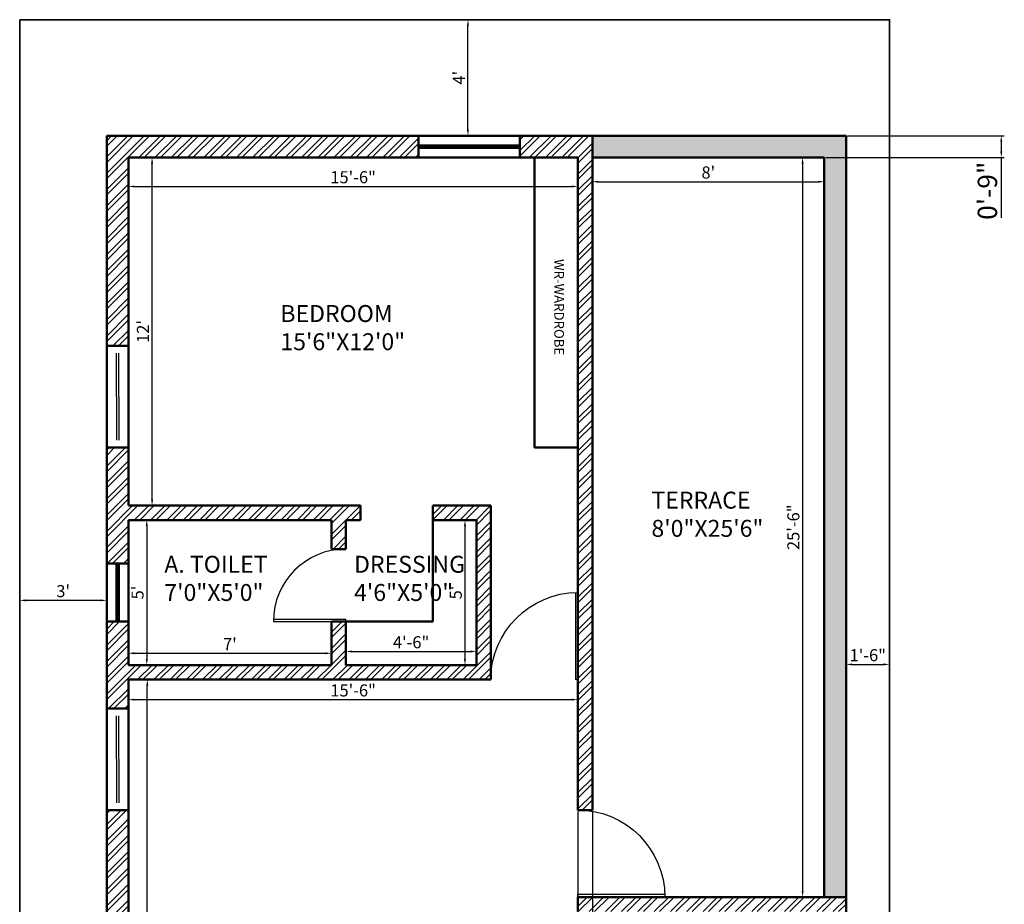
# Model space of a CAD drawing. Units: inches. Extents: x 1986 to 21484, y -1816 to 2016.
# Tile 84 of 85: x 5295 to 5702, y 1535 to 1901. Entities that reach past the tile are written whole.
import ezdxf

# ---------------------------------------------------------------- set-up
doc = ezdxf.new("R2010")
doc.units = ezdxf.units.IN
for name, color, linetype, lineweight in [('A-ANNO-DIMS', 2, 'Continuous', 18), ('A-ANNO-TEXT', 7, 'Continuous', 18), ('A-AREA-IDEN', 3, 'Continuous', 18), ('A-DOOR', 3, 'Continuous', 25), ('A-GLAZ', 4, 'Continuous', 25), ('A-WALL', 7, 'Continuous', 50), ('A-WALL-PATT', 8, 'Continuous', 13), ('C-PROP', 7, 'Continuous', 35)]:
    doc.layers.add(name, color=color, linetype=linetype, lineweight=lineweight)
doc.styles.get("Standard").update_dxf_attribs({"font": 'arial.ttf'})
doc.dimstyles.new('ISO-25', dxfattribs={"dimtxt": 8, "dimasz": 2.5, "dimexe": 1.25, "dimexo": 0.625, "dimtad": 1, "dimdec": 1, "dimlunit": 3, "dimtxsty": 'Standard', "dimcen": 2.5, "dimadec": 0, "dimazin": 0, "dimtfac": 1, "dimtdec": 1, "dimtmove": 0, "dimatfit": 3, "dimfxl": 1, "dimarcsym": 0})

# ---------------------------------------------------------------- blocks, each defined once
blk = doc.blocks.new('D2')
for p, q in [((1722.5, 1505.46), (1722.5, 1475.46)), ((1723.5, 1505.46), (1723.5, 1475.46)), ((1722.5, 1475.46), (1723.5, 1475.46))]:
    blk.add_line(p, q)
blk.add_arc((1722.5, 1475.46), 30, 0, 90)
blk = doc.blocks.new('D1')
for p, q in [((1805.96, 1500.36), (1805.96, 1464.36)), ((1806.96, 1500.36), (1806.96, 1464.36)), ((1805.96, 1464.36), (1806.96, 1464.36))]:
    blk.add_line(p, q)
blk.add_arc((1805.96, 1464.36), 36, 0, 90)
blk = doc.blocks.new('*D59')
at = {"layer": 'A-ANNO-DIMS', "color": 0, "lineweight": -2, "transparency": 16777216}
for p, q in [((5340.51, 1627.75), (5348.95, 1627.75)), ((5347.7, 1390.25), (5347.7, 1625.25)), ((5340.51, 1387.75), (5348.95, 1387.75))]:
    blk.add_line(p, q, dxfattribs=at)
at = {"layer": 'A-ANNO-DIMS', "color": 0, "transparency": 16777216}
for points in [[(5347.28, 1625.25), (5348.11, 1625.25), (5347.7, 1627.75)], [(5347.28, 1390.25), (5348.11, 1390.25), (5347.7, 1387.75)]]:
    blk.add_solid(points, dxfattribs=at)
at = {"layer": 'Defpoints', "color": 0, "transparency": 16777216}
for p in [(5339.88, 1627.75), (5347.7, 1627.75), (5339.88, 1387.75)]:
    blk.add_point(p, dxfattribs=at)
at = {"layer": 'A-ANNO-DIMS', "color": 0, "transparency": 16777216, "insert": (5344.52, 1507.75), "char_height": 5, "attachment_point": 5, "rotation": 90}
blk.add_mtext("20'", dxfattribs=at)
blk = doc.blocks.new('*D60')
at = {"layer": 'A-ANNO-DIMS', "color": 0, "lineweight": -2, "transparency": 16777216}
for p, q in [((5339.88, 1627.13), (5339.88, 1618.17)), ((5525.88, 1627.13), (5525.88, 1618.17)), ((5342.38, 1619.42), (5523.38, 1619.42))]:
    blk.add_line(p, q, dxfattribs=at)
at = {"layer": 'A-ANNO-DIMS', "color": 0, "transparency": 16777216}
for points in [[(5342.38, 1619.84), (5342.38, 1619.01), (5339.88, 1619.42)], [(5523.38, 1619.84), (5523.38, 1619.01), (5525.88, 1619.42)]]:
    blk.add_solid(points, dxfattribs=at)
at = {"layer": 'Defpoints', "color": 0, "transparency": 16777216}
for p in [(5339.88, 1627.75), (5525.88, 1627.75), (5525.88, 1619.42)]:
    blk.add_point(p, dxfattribs=at)
at = {"layer": 'A-ANNO-DIMS', "color": 0, "transparency": 16777216, "insert": (5432.88, 1622.6), "char_height": 5, "attachment_point": 5}
blk.add_mtext('15\'-6"', dxfattribs=at)
blk = doc.blocks.new('*D61')
at = {"layer": 'A-ANNO-DIMS', "color": 0, "lineweight": -2, "transparency": 16777216}
for p, q in [((5531.88, 1843.13), (5531.88, 1832.47)), ((5627.88, 1843.13), (5627.88, 1832.47)), ((5534.38, 1833.72), (5625.38, 1833.72))]:
    blk.add_line(p, q, dxfattribs=at)
at = {"layer": 'A-ANNO-DIMS', "color": 0, "transparency": 16777216}
for points in [[(5534.38, 1834.13), (5534.38, 1833.3), (5531.88, 1833.72)], [(5625.38, 1834.13), (5625.38, 1833.3), (5627.88, 1833.72)]]:
    blk.add_solid(points, dxfattribs=at)
at = {"layer": 'Defpoints', "color": 0, "transparency": 16777216}
for p in [(5531.88, 1843.75), (5627.88, 1843.75), (5627.88, 1833.72)]:
    blk.add_point(p, dxfattribs=at)
at = {"layer": 'A-ANNO-DIMS', "color": 0, "transparency": 16777216, "insert": (5579.88, 1836.89), "char_height": 5, "attachment_point": 5}
blk.add_mtext("8'", dxfattribs=at)
blk = doc.blocks.new('*D62')
at = {"layer": 'A-ANNO-DIMS', "color": 0, "lineweight": -2, "transparency": 16777216}
for p, q in [((5627.26, 1843.75), (5617.65, 1843.75)), ((5618.9, 1841.25), (5618.9, 1540.25)), ((5627.26, 1537.75), (5617.65, 1537.75))]:
    blk.add_line(p, q, dxfattribs=at)
at = {"layer": 'A-ANNO-DIMS', "color": 0, "transparency": 16777216}
for points in [[(5618.49, 1841.25), (5619.32, 1841.25), (5618.9, 1843.75)], [(5618.49, 1540.25), (5619.32, 1540.25), (5618.9, 1537.75)]]:
    blk.add_solid(points, dxfattribs=at)
at = {"layer": 'Defpoints', "color": 0, "transparency": 16777216}
for p in [(5627.88, 1843.75), (5618.9, 1537.75), (5627.88, 1537.75)]:
    blk.add_point(p, dxfattribs=at)
at = {"layer": 'A-ANNO-DIMS', "color": 0, "transparency": 16777216, "insert": (5615.73, 1690.75), "char_height": 5, "attachment_point": 5, "rotation": 90}
blk.add_mtext('25\'-6"', dxfattribs=at)
blk = doc.blocks.new('*D63')
at = {"layer": 'A-ANNO-DIMS', "color": 0, "lineweight": -2, "transparency": 16777216}
for p, q in [((5340.51, 1693.75), (5348.73, 1693.75)), ((5347.48, 1691.25), (5347.48, 1636.25)), ((5340.51, 1633.75), (5348.73, 1633.75))]:
    blk.add_line(p, q, dxfattribs=at)
at = {"layer": 'A-ANNO-DIMS', "color": 0, "transparency": 16777216}
for points in [[(5347.06, 1691.25), (5347.89, 1691.25), (5347.48, 1693.75)], [(5347.06, 1636.25), (5347.89, 1636.25), (5347.48, 1633.75)]]:
    blk.add_solid(points, dxfattribs=at)
at = {"layer": 'Defpoints', "color": 0, "transparency": 16777216}
for p in [(5339.88, 1693.75), (5339.88, 1633.75), (5347.48, 1633.75)]:
    blk.add_point(p, dxfattribs=at)
at = {"layer": 'A-ANNO-DIMS', "color": 0, "transparency": 16777216, "insert": (5344.31, 1663.75), "char_height": 5, "attachment_point": 5, "rotation": 90}
blk.add_mtext("5'", dxfattribs=at)
blk = doc.blocks.new('*D64')
at = {"layer": 'A-ANNO-DIMS', "color": 0, "lineweight": -2, "transparency": 16777216}
for p, q in [((5339.88, 1634.38), (5339.88, 1639.87)), ((5342.38, 1638.62), (5421.38, 1638.62)), ((5423.88, 1634.38), (5423.88, 1639.87))]:
    blk.add_line(p, q, dxfattribs=at)
at = {"layer": 'A-ANNO-DIMS', "color": 0, "transparency": 16777216}
for points in [[(5342.38, 1639.03), (5342.38, 1638.2), (5339.88, 1638.62)], [(5421.38, 1639.03), (5421.38, 1638.2), (5423.88, 1638.62)]]:
    blk.add_solid(points, dxfattribs=at)
at = {"layer": 'Defpoints', "color": 0, "transparency": 16777216}
for p in [(5423.88, 1638.62), (5339.88, 1633.75), (5423.88, 1633.75)]:
    blk.add_point(p, dxfattribs=at)
at = {"layer": 'A-ANNO-DIMS', "color": 0, "transparency": 16777216, "insert": (5381.88, 1641.74), "char_height": 5, "attachment_point": 5}
blk.add_mtext("7'", dxfattribs=at)
blk = doc.blocks.new('*D65')
at = {"layer": 'A-ANNO-DIMS', "color": 0, "lineweight": -2, "transparency": 16777216}
for p, q in [((5429.88, 1634.38), (5429.88, 1640.6)), ((5432.38, 1639.35), (5481.38, 1639.35)), ((5483.88, 1634.38), (5483.88, 1640.6))]:
    blk.add_line(p, q, dxfattribs=at)
at = {"layer": 'A-ANNO-DIMS', "color": 0, "transparency": 16777216}
for points in [[(5432.38, 1639.76), (5432.38, 1638.93), (5429.88, 1639.35)], [(5481.38, 1639.76), (5481.38, 1638.93), (5483.88, 1639.35)]]:
    blk.add_solid(points, dxfattribs=at)
at = {"layer": 'Defpoints', "color": 0, "transparency": 16777216}
for p in [(5483.88, 1639.35), (5429.88, 1633.75), (5483.88, 1633.75)]:
    blk.add_point(p, dxfattribs=at)
at = {"layer": 'A-ANNO-DIMS', "color": 0, "transparency": 16777216, "insert": (5456.88, 1642.53), "char_height": 5, "attachment_point": 5}
blk.add_mtext('4\'-6"', dxfattribs=at)
blk = doc.blocks.new('*D66')
at = {"layer": 'A-ANNO-DIMS', "color": 0, "lineweight": -2, "transparency": 16777216}
for p, q in [((5483.26, 1693.75), (5477.92, 1693.75)), ((5479.17, 1691.25), (5479.17, 1636.25)), ((5483.26, 1633.75), (5477.92, 1633.75))]:
    blk.add_line(p, q, dxfattribs=at)
at = {"layer": 'A-ANNO-DIMS', "color": 0, "transparency": 16777216}
for points in [[(5478.75, 1691.25), (5479.58, 1691.25), (5479.17, 1693.75)], [(5478.75, 1636.25), (5479.58, 1636.25), (5479.17, 1633.75)]]:
    blk.add_solid(points, dxfattribs=at)
at = {"layer": 'Defpoints', "color": 0, "transparency": 16777216}
for p in [(5483.88, 1693.75), (5479.17, 1633.75), (5483.88, 1633.75)]:
    blk.add_point(p, dxfattribs=at)
at = {"layer": 'A-ANNO-DIMS', "color": 0, "transparency": 16777216, "insert": (5476, 1663.75), "char_height": 5, "attachment_point": 5, "rotation": 90}
blk.add_mtext("5'", dxfattribs=at)
blk = doc.blocks.new('*D67')
at = {"layer": 'A-ANNO-DIMS', "color": 0, "lineweight": -2, "transparency": 16777216}
for p, q in [((5340.51, 1843.75), (5350.92, 1843.75)), ((5349.67, 1702.25), (5349.67, 1841.25)), ((5340.51, 1699.75), (5350.92, 1699.75))]:
    blk.add_line(p, q, dxfattribs=at)
at = {"layer": 'A-ANNO-DIMS', "color": 0, "transparency": 16777216}
for points in [[(5349.25, 1841.25), (5350.08, 1841.25), (5349.67, 1843.75)], [(5349.25, 1702.25), (5350.08, 1702.25), (5349.67, 1699.75)]]:
    blk.add_solid(points, dxfattribs=at)
at = {"layer": 'Defpoints', "color": 0, "transparency": 16777216}
for p in [(5339.88, 1843.75), (5349.67, 1843.75), (5339.88, 1699.75)]:
    blk.add_point(p, dxfattribs=at)
at = {"layer": 'A-ANNO-DIMS', "color": 0, "transparency": 16777216, "insert": (5346.53, 1771.75), "char_height": 5, "attachment_point": 5, "rotation": 90}
blk.add_mtext("12'", dxfattribs=at)
blk = doc.blocks.new('*D68')
at = {"layer": 'A-ANNO-DIMS', "color": 0, "lineweight": -2, "transparency": 16777216}
for p, q in [((5339.88, 1843.13), (5339.88, 1830.5)), ((5525.88, 1843.13), (5525.88, 1830.5)), ((5342.38, 1831.75), (5523.38, 1831.75))]:
    blk.add_line(p, q, dxfattribs=at)
at = {"layer": 'A-ANNO-DIMS', "color": 0, "transparency": 16777216}
for points in [[(5342.38, 1832.17), (5342.38, 1831.33), (5339.88, 1831.75)], [(5523.38, 1832.17), (5523.38, 1831.33), (5525.88, 1831.75)]]:
    blk.add_solid(points, dxfattribs=at)
at = {"layer": 'Defpoints', "color": 0, "transparency": 16777216}
for p in [(5339.88, 1843.75), (5525.88, 1843.75), (5525.88, 1831.75)]:
    blk.add_point(p, dxfattribs=at)
at = {"layer": 'A-ANNO-DIMS', "color": 0, "transparency": 16777216, "insert": (5432.88, 1834.93), "char_height": 5, "attachment_point": 5}
blk.add_mtext('15\'-6"', dxfattribs=at)
blk = doc.blocks.new('*D69')
at = {"layer": 'A-ANNO-DIMS', "color": 0, "lineweight": -2, "transparency": 16777216}
for p, q in [((5479.79, 1900.75), (5481.65, 1900.75)), ((5480.4, 1855.25), (5480.4, 1898.25)), ((5479.79, 1852.75), (5481.65, 1852.75))]:
    blk.add_line(p, q, dxfattribs=at)
at = {"layer": 'A-ANNO-DIMS', "color": 0, "transparency": 16777216}
for points in [[(5479.98, 1898.25), (5480.82, 1898.25), (5480.4, 1900.75)], [(5479.98, 1855.25), (5480.82, 1855.25), (5480.4, 1852.75)]]:
    blk.add_solid(points, dxfattribs=at)
at = {"layer": 'Defpoints', "color": 0, "transparency": 16777216}
for p in [(5479.17, 1900.75), (5480.4, 1900.75), (5479.17, 1852.75)]:
    blk.add_point(p, dxfattribs=at)
at = {"layer": 'A-ANNO-DIMS', "color": 0, "transparency": 16777216, "insert": (5477.28, 1876.75), "char_height": 5, "attachment_point": 5, "rotation": 90}
blk.add_mtext("4'", dxfattribs=at)
blk = doc.blocks.new('*D70')
at = {"layer": 'A-ANNO-DIMS', "color": 0, "lineweight": -2, "transparency": 16777216}
for p, q in [((5294.88, 1661.13), (5294.88, 1661.75)), ((5328.38, 1660.5), (5297.38, 1660.5)), ((5330.88, 1661.13), (5330.88, 1661.75))]:
    blk.add_line(p, q, dxfattribs=at)
at = {"layer": 'A-ANNO-DIMS', "color": 0, "transparency": 16777216}
for points in [[(5297.38, 1660.92), (5297.38, 1660.08), (5294.88, 1660.5)], [(5328.38, 1660.92), (5328.38, 1660.08), (5330.88, 1660.5)]]:
    blk.add_solid(points, dxfattribs=at)
at = {"layer": 'Defpoints', "color": 0, "transparency": 16777216}
for p in [(5294.88, 1660.5), (5294.88, 1660.5), (5330.88, 1660.5)]:
    blk.add_point(p, dxfattribs=at)
at = {"layer": 'A-ANNO-DIMS', "color": 0, "transparency": 16777216, "insert": (5312.88, 1663.68), "char_height": 5, "attachment_point": 5}
blk.add_mtext("3'", dxfattribs=at)
blk = doc.blocks.new('*D71')
at = {"layer": 'A-ANNO-DIMS', "color": 0, "lineweight": -2, "transparency": 16777216}
for p, q in [((5636.88, 1634.63), (5636.88, 1635.25)), ((5654.88, 1634.63), (5654.88, 1635.25)), ((5639.38, 1634), (5652.38, 1634))]:
    blk.add_line(p, q, dxfattribs=at)
at = {"layer": 'A-ANNO-DIMS', "color": 0, "transparency": 16777216}
for points in [[(5639.38, 1634.42), (5639.38, 1633.59), (5636.88, 1634)], [(5652.38, 1634.42), (5652.38, 1633.59), (5654.88, 1634)]]:
    blk.add_solid(points, dxfattribs=at)
at = {"layer": 'Defpoints', "color": 0, "transparency": 16777216}
for p in [(5636.88, 1634), (5654.88, 1634), (5654.88, 1634)]:
    blk.add_point(p, dxfattribs=at)
at = {"layer": 'A-ANNO-DIMS', "color": 0, "transparency": 16777216, "insert": (5645.88, 1637.18), "char_height": 5, "attachment_point": 5}
blk.add_mtext('1\'-6"', dxfattribs=at)
blk = doc.blocks.new('WIN-36')
for p, q in [((0, 36), (0, 0)), ((0, 36), (0, 0)), ((1, 36), (1, 0))]:
    blk.add_line(p, q)
blk = doc.blocks.new('*D133')
at = {"layer": 'A-ANNO-DIMS', "color": 0, "lineweight": -2, "transparency": 16777216}
for p, q in [((5637.51, 1852.75), (5702.38, 1852.75)), ((5701.13, 1850.25), (5701.13, 1846.25)), ((5628.51, 1843.75), (5702.38, 1843.75)), ((5701.13, 1843.75), (5701.13, 1818.74))]:
    blk.add_line(p, q, dxfattribs=at)
at = {"layer": 'A-ANNO-DIMS', "color": 0, "transparency": 16777216}
for points in [[(5700.72, 1850.25), (5701.55, 1850.25), (5701.13, 1852.75)], [(5700.72, 1846.25), (5701.55, 1846.25), (5701.13, 1843.75)]]:
    blk.add_solid(points, dxfattribs=at)
at = {"layer": 'Defpoints', "color": 0, "transparency": 16777216}
for p in [(5636.88, 1852.75), (5627.88, 1843.75), (5701.13, 1843.75)]:
    blk.add_point(p, dxfattribs=at)
at = {"layer": 'A-ANNO-DIMS', "color": 0, "transparency": 16777216, "insert": (5696.42, 1829.99), "char_height": 8, "attachment_point": 5, "rotation": 90}
blk.add_mtext('0\'-9"', dxfattribs=at)
blk = doc.blocks.new('*D134')
at = {"layer": 'A-ANNO-DIMS', "color": 0, "lineweight": -2, "transparency": 16777216}
for p, q in [((5525.88, 1573.13), (5525.88, 953.11)), ((5531.88, 1573.13), (5531.88, 953.11)), ((5523.38, 954.36), (5520.88, 954.36)), ((5525.88, 954.36), (5531.88, 954.36)), ((5534.38, 954.36), (5559.4, 954.36))]:
    blk.add_line(p, q, dxfattribs=at)
at = {"layer": 'A-ANNO-DIMS', "color": 0, "transparency": 16777216}
for points in [[(5523.38, 954.78), (5523.38, 953.95), (5525.88, 954.36)], [(5534.38, 954.78), (5534.38, 953.95), (5531.88, 954.36)]]:
    blk.add_solid(points, dxfattribs=at)
at = {"layer": 'Defpoints', "color": 0, "transparency": 16777216}
for p in [(5525.88, 1573.75), (5531.88, 1573.75), (5531.88, 954.36)]:
    blk.add_point(p, dxfattribs=at)
at = {"layer": 'A-ANNO-DIMS', "color": 0, "transparency": 16777216, "insert": (5548.14, 959.07), "char_height": 8, "attachment_point": 5}
blk.add_mtext('0\'-6"', dxfattribs=at)

msp = doc.modelspace()

# ---------------------------------------------------------------- hatches: boundary and pattern name
at = {"layer": 'A-WALL-PATT'}
h = msp.add_hatch(dxfattribs=at)
h.set_pattern_fill('ANSI32', color=256, scale=0.5)
h.set_pattern_definition([(45, (1297.9813, 0), (-3.367596, 3.367596), []), (45, (1300.2263, 0), (-3.367596, 3.367596), [])])
h.paths.add_polyline_path([(5459.88, 1852.75), (5330.88, 1852.75), (5330.88, 1765.75), (5339.88, 1765.75), (5339.88, 1843.75), (5459.88, 1843.75)])
h.paths.add_polyline_path([(5435.88, 1699.75), (5339.88, 1699.75), (5339.88, 1723.75), (5330.88, 1723.75), (5330.88, 1675.75), (5339.88, 1675.75), (5339.88, 1693.75), (5423.88, 1693.75), (5423.88, 1681.75), (5429.88, 1681.75), (5429.88, 1693.75), (5435.88, 1693.75)])
h.paths.add_polyline_path([(5531.88, 1852.75), (5501.88, 1852.75), (5501.88, 1843.75), (5525.88, 1843.75), (5525.88, 1573.75), (5531.88, 1573.75)])
h.paths.add_polyline_path([(5339.88, 1651.75), (5330.88, 1651.75), (5330.88, 1615.75), (5339.88, 1615.75), (5339.88, 1627.75), (5489.88, 1627.75), (5489.88, 1699.75), (5465.88, 1699.75), (5465.88, 1693.75), (5483.88, 1693.75), (5483.88, 1633.75), (5429.88, 1633.75), (5429.88, 1651.75), (5423.88, 1651.75), (5423.88, 1633.75), (5339.88, 1633.75)])
h.paths.add_polyline_path([(5339.88, 1573.75), (5330.88, 1573.75), (5330.88, 1528.77), (5339.88, 1528.77)])
h.paths.add_polyline_path([(5339.88, 1486.77), (5330.88, 1486.77), (5330.88, 1441.75), (5339.88, 1441.75)])
h.paths.add_polyline_path([(5339.88, 1399.75), (5330.88, 1399.75), (5330.88, 1258.75), (5339.88, 1258.75)])
h.paths.add_polyline_path([(5404.38, 1387.75), (5375.88, 1387.75), (5375.88, 1378.75), (5404.38, 1378.75)])
h.paths.add_polyline_path([(5471.88, 1387.75), (5446.38, 1387.75), (5446.38, 1378.75), (5462.88, 1378.75), (5462.88, 1354.75), (5471.88, 1354.75)])
h.paths.add_polyline_path([(5636.88, 1387.75), (5627.88, 1387.75), (5507.88, 1387.75), (5507.88, 1381.75), (5627.88, 1381.75), (5627.88, 1363.75), (5636.88, 1363.75)])
h.paths.add_polyline_path([(5636.88, 1495.75), (5627.88, 1495.75), (5627.88, 1477.75), (5636.88, 1477.75)])
h.paths.add_polyline_path([(5636.88, 1537.75), (5525.88, 1537.75), (5525.88, 1531.75), (5627.88, 1531.75), (5636.88, 1531.75)])
h.paths.add_polyline_path([(5636.88, 1441.75), (5627.88, 1441.75), (5627.88, 1423.75), (5636.88, 1423.75)])
h.paths.add_polyline_path([(5636.88, 1339.75), (5627.88, 1339.75), (5627.88, 1321.75), (5531.88, 1321.75), (5531.88, 1351.75), (5525.88, 1351.75), (5525.88, 1315.75), (5627.88, 1315.75), (5627.88, 1303.75), (5636.88, 1303.75)])
h.paths.add_polyline_path([(5636.88, 1261.75), (5627.88, 1261.75), (5627.88, 1189.75), (5636.88, 1189.75)])
h.paths.add_polyline_path([(5636.88, 1147.75), (5627.88, 1147.75), (5627.88, 1123.75), (5519.88, 1123.75), (5519.88, 1114.75), (5636.88, 1114.75)])
h.paths.add_polyline_path([(5471.88, 1147.75), (5462.88, 1147.75), (5462.88, 1114.75), (5477.88, 1114.75), (5477.88, 1123.75), (5471.88, 1123.75)])
h.paths.add_polyline_path([(5471.88, 1312.75), (5462.88, 1312.75), (5462.88, 1189.75), (5471.88, 1189.75)])
h = msp.add_hatch(color=256, dxfattribs=at)
h.dxf.hatch_style = 1
h.paths.add_polyline_path([(5636.88, 1852.75), (5531.88, 1852.75), (5531.88, 1843.75), (5627.88, 1843.75), (5627.88, 1537.75), (5636.88, 1537.75)])

# ---------------------------------------------------------------- linework, layer by layer
at = {"layer": 'A-WALL'}
for p, q in [((5330.88, 1852.75), (5636.88, 1852.75)), ((5330.88, 1258.75), (5330.88, 1852.75)), ((5459.88, 1843.75), (5459.88, 1852.75)), ((5501.88, 1843.75), (5501.88, 1852.75)), ((5531.88, 1852.75), (5531.88, 1573.75)), ((5636.88, 1852.75), (5636.88, 1114.75)), ((5459.88, 1848.75), (5501.88, 1848.75)), ((5459.88, 1847.75), (5501.88, 1847.75)), ((5339.88, 1843.75), (5525.88, 1843.75)), ((5339.88, 1699.75), (5339.88, 1843.75)), ((5507.88, 1843.75), (5507.88, 1723.75)), ((5525.88, 1843.75), (5525.88, 1573.75)), ((5531.88, 1843.75), (5627.88, 1843.75)), ((5627.88, 1843.75), (5627.88, 1537.75)), ((5330.88, 1765.75), (5339.88, 1765.75)), ((5330.88, 1723.75), (5339.88, 1723.75)), ((5507.88, 1723.75), (5525.88, 1723.75)), ((5339.88, 1699.75), (5435.88, 1699.75)), ((5435.88, 1699.75), (5435.88, 1693.75)), ((5465.88, 1699.75), (5489.88, 1699.75)), ((5465.88, 1699.75), (5465.88, 1651.75)), ((5489.88, 1699.75), (5489.88, 1627.75)), ((5339.88, 1693.75), (5423.88, 1693.75)), ((5339.88, 1633.75), (5339.88, 1693.75)), ((5423.88, 1681.75), (5423.88, 1693.75)), ((5429.88, 1693.75), (5435.88, 1693.75)), ((5429.88, 1681.75), (5429.88, 1693.75)), ((5465.88, 1693.75), (5483.88, 1693.75)), ((5483.88, 1693.75), (5483.88, 1633.75)), ((5423.88, 1681.75), (5429.88, 1681.75)), ((5330.88, 1675.75), (5339.88, 1675.75)), ((5334.88, 1651.75), (5334.88, 1675.75)), ((5335.88, 1651.75), (5335.88, 1675.75)), ((5330.88, 1651.75), (5339.88, 1651.75)), ((5423.88, 1633.75), (5423.88, 1651.75)), ((5423.88, 1651.75), (5465.88, 1651.75)), ((5429.88, 1633.75), (5429.88, 1651.75)), ((5339.88, 1633.75), (5423.88, 1633.75)), ((5429.88, 1633.75), (5483.88, 1633.75)), ((5339.88, 1258.75), (5339.88, 1627.75)), ((5339.88, 1627.75), (5489.88, 1627.75)), ((5330.88, 1615.75), (5339.88, 1615.75)), ((5330.88, 1573.75), (5339.88, 1573.75)), ((5525.88, 1573.75), (5531.88, 1573.75)), ((5525.88, 1537.75), (5636.88, 1537.75)), ((5525.88, 1537.75), (5525.88, 1531.75))]:
    msp.add_line(p, q, dxfattribs=at)
at = {"layer": 'C-PROP'}
msp.add_lwpolyline([(5294.88, 1900.75), (5654.88, 1900.75), (5654.88, 1066.75), (5294.88, 1066.75)], close=True, dxfattribs=at)

# ---------------------------------------------------------------- block references
at = {"layer": 'A-DOOR', "rotation": 90}
msp.add_blockref('D2', (6905.34, -70.75), dxfattribs=at)
at = {"layer": 'A-DOOR', "xscale": -1}
msp.add_blockref('D1', (7331.85, 163.39), dxfattribs=at)
at = {"layer": 'A-DOOR', "xscale": -1, "rotation": 270}
msp.add_blockref('D1', (4061.52, -268.21), dxfattribs=at)
at = {"layer": 'A-GLAZ'}
for p, rotation in [((5334.98, 1726.75), 0.302793432207276), ((5334.98, 1576.75), 0.3027934322048686)]:
    msp.add_blockref('WIN-36', p, dxfattribs=dict(at, rotation=rotation))

# ---------------------------------------------------------------- texts
at = {"layer": 'A-ANNO-TEXT', "insert": (5520.14, 1801.73), "char_height": 4, "attachment_point": 1, "rotation": 270}
msp.add_mtext_dynamic_manual_height_columns('{\\fTimes New Roman|b0|i0|c0|p18;WR-WARDROBE}', width=105.6127, gutter_width=12.5, heights=[0], dxfattribs=at)
at = {"layer": 'A-AREA-IDEN', "char_height": 7, "attachment_point": 1}
for s, insert in [('{\\fTimes New Roman|b0|i0|c0|p18;BEDROOM \\P15\'6"X12\'0"}', (5402.77, 1782.68)), ('{\\fTimes New Roman|b0|i0|c0|p18;TERRACE\\P8\'0"X25\'6"}', (5556.34, 1705.47)), ('{\\fTimes New Roman|b0|i0|c0|p18;A. TOILET\\P7\'0"X5\'0"}', (5354.74, 1678.93)), ('{\\fTimes New Roman|b0|i0|c0|p18;DRESSING\\P4\'6"X5\'0"}', (5433.27, 1678.93))]:
    msp.add_mtext_dynamic_manual_height_columns(s, width=105.6127, gutter_width=12.5, heights=[0], dxfattribs=dict(at, insert=insert))

# ---------------------------------------------------------------- dimensions: what is measured, and where the dimension line sits
at = {"layer": 'A-ANNO-DIMS'}
for base, p1, p2, angle, override, picture, middle in [((5480.4, 1900.75), (5479.17, 1852.75), (5479.17, 1900.75), 90, {"dimtxt": 5, "dimclrd": 0, "dimclre": 0, "dimclrt": 0}, '*D69', (5477.28, 1876.75)), ((5701.13, 1843.75), (5636.88, 1852.75), (5627.88, 1843.75), 90, {"dimdec": 1, "dimlfac": 1, "dimrnd": 0, "dimzin": 1, "dimdsep": 46, "dimlunit": 4, "dimfrac": 2}, '*D133', (5696.42, 1829.99)), ((5349.67, 1843.75), (5339.88, 1699.75), (5339.88, 1843.75), 270, {"dimtxt": 5, "dimclrd": 0, "dimclre": 0, "dimclrt": 0}, '*D67', (5346.53, 1771.75)), ((5618.9, 1537.75), (5627.88, 1843.75), (5627.88, 1537.75), 90, {"dimtxt": 5, "dimclrd": 0, "dimclre": 0, "dimclrt": 0}, '*D62', (5615.73, 1690.75)), ((5347.48, 1633.75), (5339.88, 1693.75), (5339.88, 1633.75), 90, {"dimtxt": 5, "dimclrd": 0, "dimclre": 0, "dimclrt": 0}, '*D63', (5344.31, 1663.75)), ((5479.17, 1633.75), (5483.88, 1693.75), (5483.88, 1633.75), 90, {"dimtxt": 5, "dimclrd": 0, "dimclre": 0, "dimclrt": 0}, '*D66', (5476, 1663.75)), ((5347.7, 1627.75), (5339.88, 1387.75), (5339.88, 1627.75), 90, {"dimtxt": 5, "dimclrd": 0, "dimclre": 0, "dimclrt": 0}, '*D59', (5344.52, 1507.75))]:
    dim = msp.add_linear_dim(base=base, p1=p1, p2=p2, angle=angle, dimstyle='ISO-25', override=override, dxfattribs=at)
    dim.commit()
    dim.dimension.update_dxf_attribs({"geometry": picture, "text_midpoint": middle})
for base, p1, p2, override, picture, middle in [((5525.88, 1831.75), (5339.88, 1843.75), (5525.88, 1843.75), {"dimtxt": 5, "dimclrd": 0, "dimclre": 0, "dimclrt": 0}, '*D68', (5432.88, 1834.93)), ((5627.88, 1833.72), (5531.88, 1843.75), (5627.88, 1843.75), {"dimtxt": 5, "dimclrd": 0, "dimclre": 0, "dimclrt": 0}, '*D61', (5579.88, 1836.89)), ((5294.88, 1660.5), (5330.88, 1660.5), (5294.88, 1660.5), {"dimtxt": 5, "dimclrd": 0, "dimclre": 0, "dimclrt": 0}, '*D70', (5312.88, 1663.68)), ((5423.88, 1638.62), (5339.88, 1633.75), (5423.88, 1633.75), {"dimtxt": 5, "dimclrd": 0, "dimclre": 0, "dimclrt": 0}, '*D64', (5381.88, 1641.74)), ((5483.88, 1639.35), (5429.88, 1633.75), (5483.88, 1633.75), {"dimtxt": 5, "dimclrd": 0, "dimclre": 0, "dimclrt": 0}, '*D65', (5456.88, 1642.53)), ((5654.88, 1634), (5636.88, 1634), (5654.88, 1634), {"dimtxt": 5, "dimclrd": 0, "dimclre": 0, "dimclrt": 0}, '*D71', (5645.88, 1637.18)), ((5525.88, 1619.42), (5339.88, 1627.75), (5525.88, 1627.75), {"dimtxt": 5, "dimclrd": 0, "dimclre": 0, "dimclrt": 0}, '*D60', (5432.88, 1622.6)), ((5531.88, 954.36), (5525.88, 1573.75), (5531.88, 1573.75), {"dimdec": 1, "dimlfac": 1, "dimrnd": 0, "dimzin": 1, "dimdsep": 46, "dimlunit": 4, "dimfrac": 2}, '*D134', (5548.14, 959.07))]:
    dim = msp.add_linear_dim(base=base, p1=p1, p2=p2, dimstyle='ISO-25', override=override, dxfattribs=at)
    dim.commit()
    dim.dimension.update_dxf_attribs({"geometry": picture, "text_midpoint": middle})

doc.saveas('drawing.dxf')
